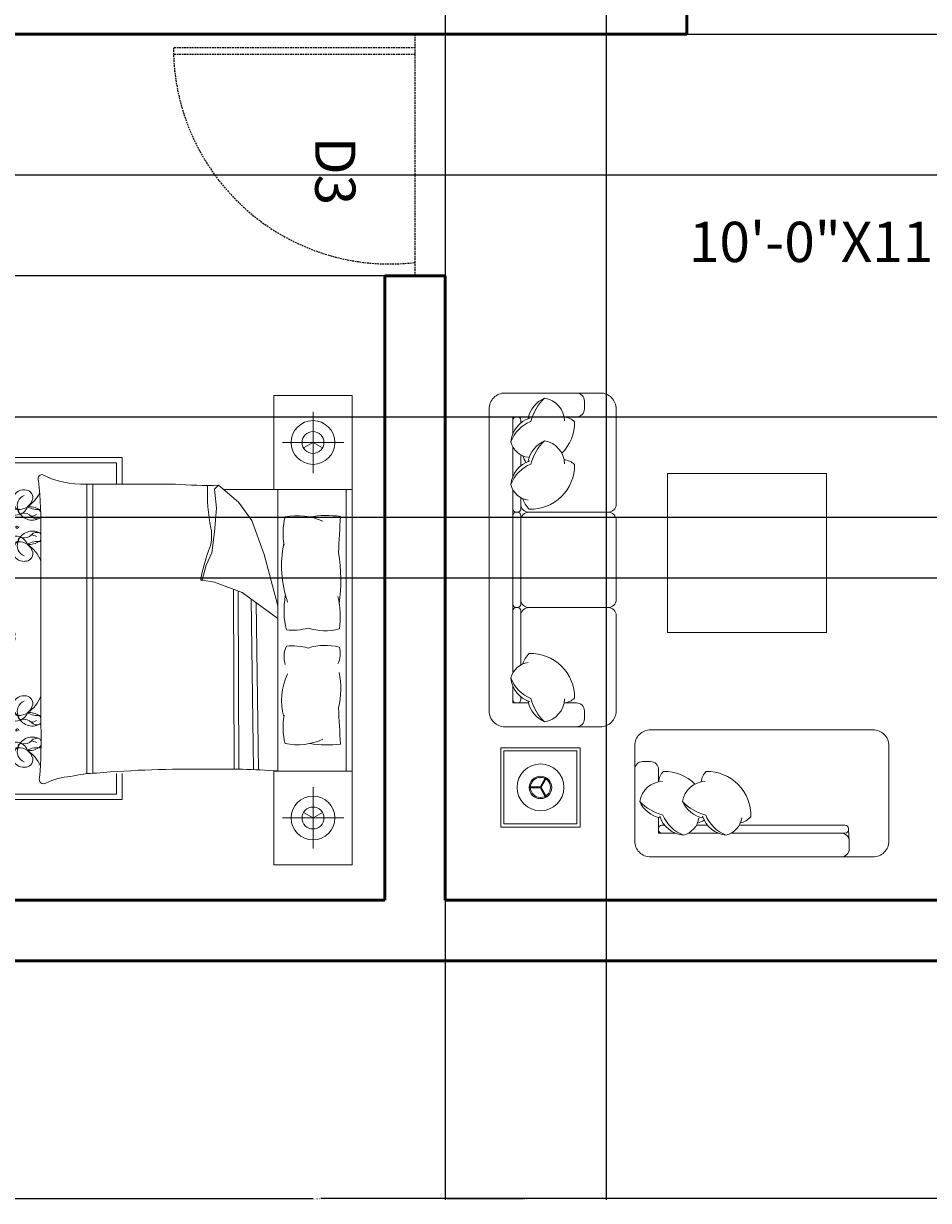
# Model space of a CAD drawing. Units: inches. Extents: x 3 to 576, y -689 to 51.
# Tile 3 of 21: x 201 to 336, y -689 to -514. Entities that reach past the tile are written whole.
import ezdxf

# ---------------------------------------------------------------- set-up
doc = ezdxf.new("R2010")
doc.units = ezdxf.units.IN
doc.header["$MEASUREMENT"] = 0
doc.linetypes.add('DASHED2', pattern=[0.375, 0.25, -0.125])
for name, color, linetype, lineweight in [('A-ANNO-DIMS', 2, 'Continuous', 18), ('A-ANNO-TEXT', 3, 'Continuous', 18), ('A-AREA-IDEN', 7, 'Continuous', 18), ('A-DOOR', 4, 'DASHED2', 25), ('A-FURN', 8, 'Continuous', 18), ('A-WALL', 7, 'Continuous', 50)]:
    doc.layers.add(name, color=color, linetype=linetype, lineweight=lineweight)
doc.styles.get("Standard").update_dxf_attribs({"font": 'arial.ttf'})
doc.dimstyles.get("Standard").update_dxf_attribs({"dimtxt": 0.18, "dimasz": 0.18, "dimexe": 0.18, "dimexo": 0.0625, "dimgap": 0.09, "dimtad": 0, "dimtih": 1, "dimtoh": 1, "dimdec": 0, "dimzin": 0, "dimdsep": 46, "dimlunit": 3, "dimtxsty": 'Standard', "dimcen": 0.09, "dimadec": 0, "dimazin": 0, "dimtfac": 1, "dimtdec": 0, "dimtofl": 0, "dimtmove": 0, "dimatfit": 3, "dimfxl": 1, "dimtolj": 1, "dimtzin": 0, "dimarcsym": 0})

# ---------------------------------------------------------------- blocks, each defined once
blk = doc.blocks.new('DAY BED1')
at = {"color": 0}
blk.add_line((0.3, 0.25), (0.225, 0.2549), dxfattribs=at)
blk.add_lwpolyline([(-0.3, 0, -0.414214), (-0.4, 0.1), (-0.4, 0.1, 0.317837), (-0.4, 0.1, -0.414214), (-0.4, 0.1), (-0.4, 0.1, 1.186185), (-0.4, 0.1, -0.414214), (-0.4, 0.1), (-0.4, 1.5, -0.414214), (-0.3, 1.6), (0.3, 1.6, -0.414214), (0.4, 1.5), (0.4, 0.1, -0.414214), (0.3, 0)], format="xyb", close=True, dxfattribs=at)
for points in [[(-0.0725, 1.45), (-0.15, 1.45, -0.414214), (-0.2, 1.5), (-0.2, 1.55, -0.414214), (-0.15, 1.6)], [(-0.0756, 1.4249, -0.356772), (0.0505, 1.5682, -0.249542), (0.1543, 1.4384, 9.61688)], [(0.0505, 1.5682, -0.14773), (0.1364, 1.422, -0.213343), (0.2624, 1.2931, -0.178662)], [(-0.0725, 1.4501, 0.165541), (-0.1386, 1.4192, 0.200231), (-0.0581, 1.2207, 0.121523)], [(0.1433, 1.4422, -0.306663), (0.2624, 1.2931, -0.30633), (0.1536, 1.1957, 0.872847)], [(0.25, 1.3448), (0.25, 1.45), (0.1517, 1.45, -0.414214)], [(0.2, 1.4118), (0.2, 1.43, -0.414214), (0.22, 1.45), (0.23, 1.45, -0.414214), (0.25, 1.43)], [(0.25, 1.43), (0.25, 1.3448, -0.414214)], [(-0.0756, 1.1556, -0.356772), (0.0505, 1.2988, -0.249542), (0.1543, 1.169, 9.61688)], [(0.0505, 1.2988, -0.14773), (0.1364, 1.1527, -0.213343), (0.2624, 1.0238, -0.178662)], [(0.25, 1.2616), (0.25, 1.0755, -0.414214)], [(0.1678, 1.1631, 0.071865), (0.1873, 1.205, -7.115464)], [(0.2, 1.1425), (0.2, 1.2113, -0.414214)], [(-0.0725, 1.1808, 0.165541), (-0.1386, 1.1498, 0.425989), (0.1479, 0.869, 0.121523), (0.1873, 0.9357, -7.115464)], [(0.1433, 1.1729, -0.306663), (0.2624, 1.0238, -0.30633), (0.1536, 0.9263, 0.872847)], [(0.25, 0.9923), (0.25, 0.2749, -0.414214), (0.23, 0.2549), (0.22, 0.2549, -0.414214), (0.2, 0.2749), (0.2, 0.9419, -0.414214)], [(0.25, 0.3775), (0.25, 0.3, 0.414214), (0.3, 0.25), (0.35, 0.25, 0.414214), (0.4, 0.3)]]:
    blk.add_lwpolyline(points, format="xyb", dxfattribs=at)
for points in [[(0.25, 1.0755), (0.25, 1.2616)], [(0.25, 0.3775), (0.25, 0.9923)]]:
    blk.add_lwpolyline(points, dxfattribs=at)
blk = doc.blocks.new('BED-DOUBLE')
for p, q in [((59.45, 69.91), (59.45, 0)), ((53.63, 58.35), (53.63, 67.49)), ((49.06, 62.92), (58.2, 62.92)), ((0, 60.68), (25.18, 60.68)), ((0, 9.72), (0, 60.68)), ((0.81, 59.87), (0.81, 10.53)), ((24.37, 59.87), (0.81, 59.87)), ((24.37, 56.73), (24.37, 59.87)), ((25.18, 60.68), (25.18, 56.73)), ((19.95, 13.6), (19.95, 56.73)), ((20.82, 13.66), (20.82, 56.73)), ((38.97, 55.99), (39.54, 56.55)), ((39.54, 56.55), (42.51, 54.01)), ((39.25, 53.16), (38.97, 55.99)), ((59.45, 55.93), (40.27, 55.93)), ((48.41, 55.93), (48.41, 13.98)), ((58.56, 13.98), (58.56, 55.93)), ((7.9, 52.98), (8.69, 53.14)), ((38.97, 49.62), (39.25, 53.16)), ((42.51, 54.01), (44.49, 51.31)), ((44.49, 51.31), (46.33, 46.22)), ((13.08, 20.76), (13.08, 49.15)), ((38.55, 46.5), (38.97, 49.62)), ((7.9, 48.1), (8.69, 47.94)), ((37.7, 44.66), (38.55, 46.5)), ((46.33, 46.22), (48.41, 38.59)), ((37.13, 42.39), (37.7, 44.66)), ((38.97, 42.11), (37.13, 42.39)), ((43.07, 40.55), (38.97, 42.11)), ((41.87, 14.23), (41.76, 41.05)), ((42.58, 14.23), (42.48, 40.78)), ((48.41, 36.72), (43.07, 40.55)), ((44.78, 14.2), (44.43, 39.58)), ((45.5, 14.17), (45.15, 39.06)), ((7.9, 22.3), (8.69, 22.46)), ((7.9, 17.41), (8.69, 17.26)), ((24.37, 10.53), (24.37, 13.61)), ((25.18, 13.59), (25.18, 9.72)), ((0.81, 10.53), (24.37, 10.53)), ((53.63, 11.56), (53.63, 2.42)), ((25.18, 9.72), (0, 9.72)), ((49.06, 6.99), (58.2, 6.99))]:
    blk.add_line(p, q)
for points in [[(47.8, 55.93), (47.8, 69.91), (59.45, 69.91)], [(53.63, 62.92), (52.22, 62.1)], [(53.63, 62.92), (55.04, 62.1)], [(59.45, 13.98), (47.8, 13.98), (47.8, 0), (59.45, 0)], [(53.63, 6.99), (52.22, 7.81)], [(53.63, 6.99), (55.04, 7.81)]]:
    blk.add_lwpolyline(points)
for points in [[(33.13, 56.7, 0.001242), (19.87, 56.73, -0.127202), (13.26, 58.14)], [(57.71, 51.91, 0.074897), (53.14, 51.83, -0.472817)], [(52.89, 35.28, 0.14099), (57.55, 35.14, 0.235245)], [(52.89, 32.3, -0.14099), (57.55, 32.44, -0.235245)], [(57.71, 18, -0.074897), (53.14, 18.08, 0.472817)], [(21.37, 13.68, 0.056112), (17.53, 13.18, 0.095341), (13.82, 12.19)]]:
    blk.add_lwpolyline(points, format="xyb")
for centre, radius in [((53.63, 62.92), 3.26), ((53.63, 62.92), 1.63), ((3.49, 50.11), 0.178), ((5.36, 48.94), 0.178), ((5.36, 21.45), 0.178), ((3.49, 20.29), 0.178), ((53.63, 6.99), 3.26), ((53.63, 6.99), 1.63)]:
    blk.add_circle(centre, radius)
for centre, radius, start, end in [((-2.47, 63.69), 5.54, 306.3036, 316.4814), ((-1.64, 62.09), 4.45, 303.4617, 330.1116), ((-0.42, 66.67), 9.13, 277.745, 311.8856), ((-1.32, 51.05), 9.13, 34.3865, 68.5908), ((13.3, 57.49), 0.645, 93.98, 207.3412), ((-0.61, 59.6), 3.71, 292.5547, 318.9546), ((1.38, 69.77), 12.63, 267.4081, 273.6519), ((6, 55.22), 1.01, 77.7115, 159.0387), ((5.45, 56.23), 0.762, 238.4633, 358.2869), ((7.95, 54.69), 2.31, 138.8402, 177.9352), ((6.56, 55.55), 0.747, 117.6827, 223.7762), ((6.39, 55.47), 0.757, 2.9516, 103.728), ((12.45, 57.59), 6.39, 192.5173, 207.1824), ((5.37, 55.04), 1.44, 345.4653, 54.2343), ((7.54, 57.02), 1.56, 211.3827, 255.2969), ((-59.69, 49.98), 72.78, 359.3433, 5.6887), ((37.8, 120.65), 64.12, 265.8294, 271.553), ((64.29, 55.36), 26.39, 177.4519, 191.3392), ((5.76, 54.77), 0.113, 177.9352, 11.4834), ((5.81, 54.78), 0.0551, 11.4834, 127.9409), ((6.09, 55.1), 0.0988, 223.7762, 159.7183), ((7.84, 54.58), 1.05, 350.264, 160.8688), ((8.16, 54.83), 1.31, 175.969, 254.3045), ((6.7, 54.8), 0.643, 333.9755, 53.2681), ((6.41, 53.42), 1.4, 6.1662, 51.5825), ((10.15, 56.66), 3.3, 211.2614, 251.7045), ((10.53, 54.2), 1.67, 84.9449, 172.8857), ((10.9, 54.49), 2.03, 182.3591, 234.0401), ((11.17, 53.54), 1.62, 111.5819, 201.4221), ((9.83, 55.04), 2.1, 265.2933, 346.921), ((10.7, 54.68), 1.18, 354.4856, 91.0538), ((8.16, 57.76), 5.29, 303.6671, 333.2997), ((9.88, 56.69), 3.75, 236.2883, 266.5076), ((9.4, 53.85), 1.74, 209.9085, 343.1337), ((10.13, 52.75), 0.434, 167.3041, 285.1471), ((11.31, 50.67), 2.7, 122.7011, 126.3445), ((11.81, 53.58), 2.23, 199.2822, 299.1751), ((12.57, 55.82), 2.9, 238.8218, 279.1554), ((11.31, 50.67), 2.7, 55.785, 94.7304), ((12.31, 52.24), 0.842, 30.0293, 52.325), ((3.75, 51.26), 0.199, 124.3538, 214.3923), ((4.04, 51.23), 0.464, 190.3057, 287.1958), ((4.17, 51.39), 0.538, 176.9701, 248.2913), ((8.01, 54.23), 5.2, 212.6784, 216.3746), ((3.99, 51.27), 0.206, 216.3746, 291.7548), ((2.83, 48.01), 3.1, 63.7819, 68.2913), ((4.48, 51.12), 0.464, 122.8155, 187.3992), ((4.12, 50.93), 0.155, 289.3605, 111.7548), ((4.24, 50.93), 0.155, 221.8703, 44.2646), ((4.69, 51.06), 0.538, 109.4799, 177.6828), ((4.4, 51.4), 0.199, 56.8636, 146.9021), ((4.5, 51.18), 0.206, 148.8844, 224.2646), ((8.78, 48.6), 5.2, 145.1882, 148.8844), ((5.81, 48.38), 2.9, 94.756, 119.2041), ((11.99, 44.2), 9.55, 132.2412, 142.1744), ((7.17, 51.8), 1.97, 178.3264, 187.1302), ((5.04, 51.53), 0.367, 11.3256, 64.4621), ((6.29, 52.06), 1.1, 190.2588, 210.656), ((5.55, 51.61), 0.336, 188.3432, 274.2869), ((5.84, 51.79), 0.586, 210.656, 242.6341), ((6.28, 52.3), 1.12, 218.2101, 226.3071), ((5.45, 51.35), 0.142, 325.7657, 67.4417), ((1.03, 56.11), 6.64, 313.1541, 322.0459), ((5.96, 45.49), 5.79, 73.5842, 93.8277), ((5.91, 52.13), 0.137, 142.4737, 265.053), ((6.09, 52.15), 0.294, 127.7621, 169.0403), ((5.94, 52.4), 0.414, 265.053, 338.3618), ((6.48, 51.84), 0.541, 113.4276, 137.6104), ((6.42, 52.4), 0.178, 183.2768, 356.7232), ((6.55, 52.07), 0.291, 139.7889, 227.6792), ((6.46, 51.97), 0.153, 227.6792, 350.3487), ((5.87, 52.08), 0.583, 353.0852, 15.7171), ((6.25, 52.01), 0.368, 350.3487, 43.6538), ((6.93, 52.39), 0.428, 198.7263, 262.5032), ((6.59, 52.19), 0.17, 1.1081, 91.8675), ((6.91, 52.1), 0.138, 255.2356, 54.9248), ((6.7, 52.15), 0.297, 11.5637, 52.6358), ((9.52, 51.39), 1.97, 178.3264, 187.1302), ((7.39, 51.11), 0.367, 11.3256, 64.4621), ((8.64, 51.64), 1.1, 190.2588, 210.656), ((7.9, 51.19), 0.336, 188.3432, 274.2869), ((8.19, 51.38), 0.586, 210.656, 242.6341), ((8.64, 51.88), 1.12, 218.2101, 226.3071), ((7.81, 50.93), 0.142, 325.7657, 67.4417), ((8.21, 50.67), 0.336, 147.5332, 233.4768), ((7.94, 50.71), 0.142, 354.3784, 96.0543), ((8.51, 50.85), 0.586, 179.1859, 211.164), ((5.96, 45.49), 5.79, 63.0032, 69.8941), ((10.62, 50.95), 1.43, 41.5653, 105.1471), ((11.41, 53.92), 2.01, 277.436, 299.9149), ((12.48, 52.59), 1.05, 221.5653, 293.8354), ((12.31, 52.24), 0.842, 314.4517, 333.558), ((58.53, 49.42), 9.37, 165.1039, 191.0369), ((51.31, 43.01), 9.01, 65.1316, 101.7583), ((723.03, 13.38), 666.43, 176.68521, 177.14978), ((2.98, 49.84), 0.137, 142.4737, 265.053), ((3.16, 49.87), 0.294, 61.2196, 169.0403), ((3, 50.12), 0.414, 265.053, 338.3618), ((3.35, 50.47), 0.351, 157.4086, 261.4386), ((3.15, 50.48), 0.176, 58.0499, 135.6268), ((3.55, 49.55), 0.541, 113.4276, 137.6104), ((3.34, 50.37), 0.118, 172.906, 277.132), ((2.95, 50.16), 0.561, 14.7558, 58.0499), ((3.62, 49.79), 0.291, 139.7889, 227.6792), ((3.53, 49.68), 0.153, 227.6792, 350.3487), ((3.74, 50.31), 0.243, 36.1046, 181.4281), ((2.93, 49.79), 0.583, 353.0852, 15.7171), ((3.31, 49.72), 0.368, 350.3487, 43.6538), ((3.59, 50.5), 0.245, 270.0645, 331.1507), ((3.8, 50.44), 0.28, 221.8413, 265.7877), ((4, 50.1), 0.428, 198.7263, 262.5032), ((3.66, 49.9), 0.17, 1.1081, 91.8675), ((3.8, 50.33), 0.174, 263.7526, 41.7054), ((3.76, 49.86), 0.297, 11.5637, 86.365), ((5.81, 48.38), 2.9, 124.0033, 132.4917), ((3.98, 49.81), 0.138, 255.2356, 54.9248), ((4.48, 50.4), 0.493, 128.3208, 208.8162), ((4.57, 50.43), 0.59, 207.7043, 254.3516), ((4.94, 50.48), 0.812, 157.2305, 229.0635), ((4.67, 50.75), 0.478, 174.4544, 220.6188), ((4.19, 50.1), 0.812, 270.278, 342.111), ((4.73, 49.08), 0.574, 98.7227, 159.3375), ((4.44, 49.82), 0.59, 244.9899, 291.6373), ((1.96, 48.08), 3.48, 30.544, 49.818), ((3.87, 50.06), 0.574, 340.0041, 40.6188), ((4.57, 50.12), 0.478, 278.7227, 324.8872), ((4.49, 49.73), 0.493, 290.5253, 358.5375), ((5.23, 49.31), 0.351, 157.4086, 261.4386), ((5.03, 49.32), 0.176, 58.0499, 135.6268), ((5.45, 49.87), 0.493, 182.8499, 266.1226), ((5.26, 50.22), 0.478, 231.7607, 277.9252), ((5.63, 50.31), 0.812, 214.5369, 286.3699), ((5.21, 49.21), 0.118, 172.906, 277.132), ((4.83, 48.99), 0.561, 14.7558, 58.0499), ((1.96, 48.08), 3.48, 23.0501, 23.8477), ((5.4, 49.18), 0.574, 37.3105, 97.9252), ((5.61, 49.14), 0.243, 36.1046, 181.4281), ((5.47, 49.97), 0.59, 265.0106, 311.658), ((5.47, 49.33), 0.245, 270.0645, 331.1507), ((5.68, 49.17), 0.174, 263.7526, 41.7054), ((8.95, 51.12), 1.1, 211.164, 231.5612), ((9.15, 52.01), 1.97, 234.6898, 243.4936), ((9.16, 51), 1.12, 195.5129, 203.6099), ((7.9, 50.27), 0.367, 357.3579, 50.4944), ((9.48, 50.34), 0.135, 12.7051, 190.4384), ((9.56, 50.36), 0.219, 190.4384, 10.4136), ((11.81, 47.5), 2.23, 60.8249, 160.7178), ((10.62, 50.13), 1.43, 254.8529, 318.4347), ((11.41, 47.16), 2.01, 60.0851, 82.564), ((12.48, 48.49), 1.05, 66.1646, 138.4347), ((12.31, 48.84), 0.842, 23.229, 45.5483), ((32.84, 49.05), 5.69, 336.2616, 11.3392), ((4.85, 48.67), 0.137, 142.4737, 265.053), ((5.03, 48.7), 0.294, 61.2196, 169.0403), ((4.88, 48.95), 0.414, 265.053, 338.3618), ((5.43, 48.38), 0.541, 113.4276, 137.6104), ((5.5, 48.62), 0.291, 139.7889, 227.6792), ((5.4, 48.52), 0.153, 227.6792, 350.3487), ((4.81, 48.63), 0.583, 353.0852, 15.7171), ((1.96, 48.08), 3.48, 357.1071, 4.7585), ((5.19, 48.56), 0.368, 350.3487, 43.6538), ((5.68, 49.27), 0.28, 221.8413, 265.7877), ((5.87, 48.94), 0.428, 198.7263, 262.5032), ((5.53, 48.74), 0.17, 1.1081, 91.8675), ((5.64, 48.7), 0.297, 11.5637, 86.365), ((5.85, 48.65), 0.138, 255.2356, 54.9248), ((8.16, 46.25), 1.31, 105.6955, 184.031), ((6.41, 47.66), 1.4, 308.4175, 353.8338), ((10.15, 44.42), 3.3, 108.2955, 148.7386), ((9.88, 44.39), 3.75, 93.4924, 123.7117), ((9.4, 47.23), 1.74, 16.8663, 150.0915), ((10.9, 46.59), 2.03, 125.9599, 177.6409), ((11.17, 47.54), 1.62, 158.5779, 248.4181), ((9.83, 46.04), 2.1, 13.079, 94.7067), ((10.13, 48.33), 0.434, 74.8529, 192.6959), ((11.31, 50.41), 2.7, 233.6555, 237.2989), ((12.57, 45.26), 2.9, 79.7133, 121.1782), ((11.31, 50.41), 2.7, 265.2696, 304.215), ((8.16, 43.32), 5.29, 21.4941, 56.3329), ((12.31, 48.84), 0.842, 307.675, 336.7144), ((65.19, 44.49), 16.25, 168.0397, 199.2615), ((5.45, 44.85), 0.762, 1.7131, 121.5367), ((5.76, 46.31), 0.113, 348.5166, 182.0648), ((7.95, 46.39), 2.31, 182.0648, 221.1598), ((5.81, 46.3), 0.0551, 232.0591, 348.5166), ((6.56, 45.54), 0.747, 136.2238, 242.3173), ((6.13, 45.97), 0.0595, 200.2667, 136.2271), ((5.37, 46.05), 1.44, 305.7657, 14.5347), ((12.45, 43.49), 6.39, 152.8176, 167.4827), ((7.84, 46.5), 1.05, 199.1312, 9.736), ((6.7, 46.28), 0.643, 306.7319, 26.0245), ((10.53, 46.88), 1.67, 187.1143, 275.0551), ((10.7, 46.4), 1.18, 268.9462, 5.5144), ((63.55, 37.54), 27.11, 160.1194, 169.3383), ((32.41, 42.33), 25.35, 352.2196, 9.497), ((-0.61, 41.48), 3.71, 41.0454, 67.4453), ((1.38, 31.32), 12.63, 86.3481, 92.5919), ((-1.32, 50.03), 9.13, 291.4092, 325.6135), ((6, 45.86), 1.01, 200.9613, 282.2885), ((6.39, 45.61), 0.757, 256.272, 357.0484), ((7.54, 44.06), 1.56, 104.7031, 148.6173), ((-0.42, 34.41), 9.13, 4.4623, 82.255), ((-1.64, 38.99), 4.45, 1.272, 56.5383), ((37.07, 42.55), 0.169, 178.8623, 289.7536), ((-2.47, 37.39), 5.54, 17.8504, 53.6964), ((-4.03, 34.48), 8.25, 34.0123, 54.053), ((-3.99, 37.66), 5.02, 343.5431, 17.0202), ((-5.31, 35.11), 9.13, 4.4623, 27.4146), ((61.64, 37.91), 12.33, 169.8617, 193.6238), ((45.23, 36.98), 12.46, 351.5249, 13.96), ((-6.58, 35.67), 7.42, 4.3787, 5.6357), ((-11.66, 31.77), 13.27, 19.7217, 19.9028), ((3.11, 35.07), 1.01, 47.7873, 129.1145), ((3.14, 36.22), 0.762, 208.5391, 328.3627), ((4.54, 33.64), 2.31, 108.9159, 148.011), ((3.76, 35.07), 0.747, 87.7585, 193.852), ((9.89, 33.91), 6.39, 162.593, 177.2582), ((2.48, 35.23), 1.44, 315.5411, 24.3101), ((5.35, 35.86), 1.56, 181.4585, 225.3727), ((3.58, 35.09), 0.757, 333.0274, 73.8037), ((8, 34.37), 1.01, 47.7873, 129.1145), ((8.03, 35.52), 0.762, 208.5391, 328.3627), ((9.43, 32.94), 2.31, 108.9159, 148.011), ((8.65, 34.38), 0.747, 87.7585, 193.852), ((7.37, 34.53), 1.44, 315.5411, 24.3101), ((14.78, 33.21), 6.39, 162.593, 177.2582), ((8.47, 34.4), 0.757, 333.0274, 73.8037), ((10.24, 35.16), 1.56, 181.4585, 225.3727), ((50.55, 43.52), 8.57, 264.0129, 285.8293), ((2.68, 34.8), 0.113, 148.011, 341.5592), ((2.68, 33.27), 0.113, 18.4408, 211.989), ((2.73, 34.78), 0.0551, 341.5592, 98.0167), ((3.13, 34.92), 0.0988, 193.852, 129.9245), ((9.89, 34.16), 6.39, 182.7418, 197.407), ((2.48, 32.84), 1.44, 335.6899, 44.4589), ((5.35, 32.21), 1.56, 134.6273, 178.5415), ((3.58, 32.97), 0.757, 286.1963, 26.9726), ((7.57, 34.1), 0.113, 148.011, 341.5592), ((7.57, 33.97), 0.113, 18.4408, 211.989), ((9.43, 35.13), 2.31, 211.989, 251.0841), ((7.62, 34.08), 0.0551, 341.5592, 98.0167), ((7.62, 33.99), 0.0551, 261.9833, 18.4408), ((8.65, 33.69), 0.747, 166.148, 272.2415), ((8.02, 34.22), 0.0988, 193.852, 129.9245), ((8.06, 33.86), 0.0595, 230.1909, 166.0209), ((7.37, 33.54), 1.44, 335.6899, 44.4589), ((14.78, 34.86), 6.39, 182.7418, 197.407), ((8.47, 33.67), 0.757, 286.1963, 26.9726), ((10.24, 32.91), 1.56, 134.6273, 178.5415), ((1.69, 33.95), 7.07, 262.8636, 351.8197), ((-3.99, 30.4), 5.02, 342.9798, 16.4569), ((-6.58, 32.39), 7.42, 354.3643, 355.6213), ((-11.66, 36.3), 13.27, 340.0972, 340.2783), ((3.14, 31.85), 0.762, 31.6373, 151.4609), ((3.11, 33), 1.01, 230.8855, 312.2127), ((4.54, 34.43), 2.31, 211.989, 251.0841), ((2.73, 33.29), 0.0551, 261.9833, 18.4408), ((-5.31, 32.96), 9.13, 332.5854, 355.5377), ((3.76, 32.99), 0.747, 166.148, 272.2415), ((3.17, 33.16), 0.0595, 230.1909, 166.0209), ((8.03, 32.55), 0.762, 31.6373, 151.4609), ((8, 33.7), 1.01, 230.8855, 312.2127), ((53.02, 31.01), 3.71, 155.0183, 198.5407), ((50.55, 24.06), 8.57, 74.1707, 95.9871), ((54.23, 31.48), 3.46, 333.3437, 16.1026), ((2.33, 33.04), 4.09, 248.117, 276.6195), ((1.2, 29.29), 1.64, 256.3898, 349.0739), ((1.42, 30.52), 2.07, 252.8609, 311.9049), ((-1.32, 20.37), 9.13, 34.3865, 68.5908), ((57.84, 24.53), 8.9, 153.8761, 196.1746), ((45.48, 26.29), 12.29, 346.3427, 11.1841), ((1.38, 39.08), 12.63, 267.4081, 273.6519), ((-0.61, 28.92), 3.71, 292.5547, 318.9546), ((6, 24.53), 1.01, 77.7115, 159.0387), ((5.45, 25.55), 0.762, 238.4633, 358.2869), ((7.95, 24), 2.31, 138.8402, 177.9352), ((6.56, 24.86), 0.747, 117.6827, 223.7762), ((6.39, 24.79), 0.757, 2.9516, 103.728), ((7.54, 26.34), 1.56, 211.3827, 255.2969), ((5.37, 24.35), 1.44, 345.4653, 54.2343), ((12.45, 26.91), 6.39, 192.5173, 207.1824), ((7.84, 23.9), 1.05, 350.264, 160.8688), ((6.7, 24.12), 0.643, 333.9755, 53.2681), ((10.53, 23.52), 1.67, 84.9449, 172.8857), ((10.7, 24), 1.18, 354.4856, 91.0538), ((8.16, 27.08), 5.29, 303.6671, 338.5059), ((5.76, 24.08), 0.113, 177.9352, 11.4834), ((5.81, 24.09), 0.0551, 11.4834, 127.9409), ((6.09, 24.41), 0.0988, 223.7762, 159.7183), ((8.16, 24.15), 1.31, 175.969, 254.3045), ((6.41, 22.74), 1.4, 6.1662, 51.5825), ((10.15, 25.98), 3.3, 211.2614, 251.7045), ((9.88, 26.01), 3.75, 236.2883, 266.5076), ((10.9, 23.81), 2.03, 182.3591, 234.0401), ((11.17, 22.86), 1.62, 111.5819, 201.4221), ((9.83, 24.36), 2.1, 265.2933, 346.921), ((723.03, 56.53), 666.43, 182.85022, 183.31479), ((4.44, 20.58), 0.59, 68.3627, 115.0101), ((4.19, 20.3), 0.812, 17.889, 89.722), ((4.73, 21.32), 0.574, 200.6625, 261.2773), ((4.49, 20.66), 0.493, 1.4625, 69.4747), ((4.85, 21.72), 0.137, 94.947, 217.5263), ((5.03, 21.7), 0.294, 190.9597, 298.7804), ((4.88, 21.45), 0.414, 21.6382, 94.947), ((5.23, 21.09), 0.351, 98.5614, 202.5914), ((5.43, 22.01), 0.541, 222.3896, 246.5724), ((5.21, 21.19), 0.118, 82.868, 187.094), ((4.83, 21.41), 0.561, 301.9501, 345.2442), ((5.5, 21.78), 0.291, 132.3208, 220.2111), ((5.4, 21.88), 0.153, 9.6513, 132.3208), ((4.81, 21.77), 0.583, 344.2829, 6.9148), ((5.61, 21.26), 0.243, 178.5719, 323.8954), ((1.96, 22.32), 3.48, 355.2415, 2.8929), ((5.19, 21.84), 0.368, 316.3462, 9.6513), ((5.87, 21.46), 0.428, 97.4968, 161.2737), ((5.68, 21.12), 0.28, 94.2123, 138.1587), ((5.47, 21.07), 0.245, 28.8493, 89.9355), ((5.53, 21.66), 0.17, 268.1325, 358.8919), ((5.64, 21.7), 0.297, 273.635, 348.4363), ((5.68, 21.23), 0.174, 318.2946, 96.2474), ((5.85, 21.75), 0.138, 305.0752, 104.7644), ((9.4, 23.17), 1.74, 209.9085, 343.1337), ((10.13, 22.07), 0.434, 167.3041, 285.1471), ((11.31, 19.99), 2.7, 122.7011, 126.3445), ((11.81, 22.9), 2.23, 199.2822, 299.1751), ((10.62, 20.26), 1.43, 41.5653, 105.1471), ((12.57, 25.14), 2.9, 238.8218, 280.2867), ((11.31, 19.99), 2.7, 55.785, 94.7304), ((11.41, 23.23), 2.01, 277.436, 299.9149), ((12.48, 21.91), 1.05, 221.5653, 293.8354), ((12.31, 21.55), 0.842, 23.2856, 52.325), ((12.31, 21.55), 0.842, 314.4517, 336.7144), ((58.53, 20.49), 9.37, 168.9631, 194.8961), ((2.98, 20.56), 0.137, 94.947, 217.5263), ((3.16, 20.53), 0.294, 190.9597, 298.7804), ((3, 20.28), 0.414, 21.6382, 94.947), ((3.35, 19.93), 0.351, 98.5614, 202.5914), ((3.15, 19.91), 0.176, 224.3732, 301.9501), ((3.55, 20.85), 0.541, 222.3896, 246.5724), ((3.34, 20.03), 0.118, 82.868, 187.094), ((2.95, 20.24), 0.561, 301.9501, 345.2442), ((3.62, 20.61), 0.291, 132.3208, 220.2111), ((3.53, 20.71), 0.153, 9.6513, 132.3208), ((2.93, 20.61), 0.583, 344.2829, 6.9148), ((3.74, 20.09), 0.243, 178.5719, 323.8954), ((3.31, 20.68), 0.368, 316.3462, 9.6513), ((4.04, 19.17), 0.464, 72.8042, 169.6943), ((4, 20.3), 0.428, 97.4968, 161.2737), ((3.8, 19.96), 0.28, 94.2123, 138.1587), ((3.59, 19.9), 0.245, 28.8493, 89.9355), ((4.17, 19.01), 0.538, 111.7087, 183.0299), ((3.66, 20.5), 0.17, 268.1325, 358.8919), ((3.76, 20.54), 0.297, 273.635, 348.4363), ((3.8, 20.07), 0.174, 318.2946, 96.2474), ((3.99, 19.13), 0.206, 68.2452, 143.6254), ((5.81, 22.02), 2.9, 227.5083, 235.9967), ((3.98, 20.59), 0.138, 305.0752, 104.7644), ((2.83, 22.39), 3.1, 291.7087, 296.2181), ((4.48, 20), 0.493, 151.1838, 231.6792), ((4.48, 19.27), 0.464, 172.6008, 237.1845), ((4.57, 19.96), 0.59, 105.6484, 152.2957), ((4.12, 19.47), 0.155, 248.2452, 70.6395), ((4.94, 19.92), 0.812, 130.9365, 202.7695), ((4.24, 19.47), 0.155, 315.7354, 138.1297), ((4.69, 19.33), 0.538, 182.3172, 250.5201), ((4.67, 19.65), 0.478, 139.3812, 185.5456), ((1.96, 22.32), 3.48, 310.182, 329.456), ((4.5, 19.21), 0.206, 135.7354, 211.1156), ((3.87, 20.33), 0.574, 319.3812, 19.9959), ((5.81, 22.02), 2.9, 240.7959, 265.244), ((11.99, 26.2), 9.55, 217.8256, 227.7588), ((4.57, 20.28), 0.478, 35.1128, 81.2773), ((5.03, 21.08), 0.176, 224.3732, 301.9501), ((5.45, 20.52), 0.493, 93.8774, 177.1501), ((5.63, 20.09), 0.812, 73.6301, 145.4631), ((5.26, 20.18), 0.478, 82.0748, 128.2393), ((1.96, 22.32), 3.48, 336.1523, 336.9499), ((5.4, 21.22), 0.574, 262.0748, 322.6895), ((5.47, 20.43), 0.59, 48.342, 94.9894), ((5.96, 24.9), 5.79, 266.1723, 286.4158), ((8.64, 18.76), 1.1, 149.344, 169.7412), ((7.9, 19.21), 0.336, 85.7131, 171.6568), ((8.19, 19.02), 0.586, 117.3659, 149.344), ((8.64, 18.52), 1.12, 133.6929, 141.7899), ((7.81, 19.46), 0.142, 292.5583, 34.2343), ((8.21, 19.72), 0.336, 126.5232, 212.4668), ((8.51, 19.55), 0.586, 148.836, 180.8141), ((7.94, 19.68), 0.142, 263.9457, 5.6216), ((5.96, 24.9), 5.79, 290.1059, 296.9968), ((8.95, 19.28), 1.1, 128.4388, 148.836), ((9.15, 18.38), 1.97, 116.5064, 125.3102), ((9.16, 19.4), 1.12, 156.3901, 164.4871), ((7.9, 20.13), 0.367, 309.5056, 2.6421), ((9.56, 20.04), 0.219, 349.5864, 169.5616), ((9.48, 20.06), 0.135, 169.5616, 347.2949), ((-54.91, 18.62), 68.03, 355.2402, 1.8035), ((3.75, 19.14), 0.199, 145.6077, 235.6462), ((8.01, 16.17), 5.2, 143.6254, 147.3216), ((4.4, 18.99), 0.199, 213.0979, 303.1364), ((8.78, 21.8), 5.2, 211.1156, 214.8118), ((6.29, 18.34), 1.1, 149.344, 169.7412), ((7.17, 18.6), 1.97, 172.8698, 181.6736), ((5.04, 18.87), 0.367, 295.5379, 348.6744), ((5.55, 18.79), 0.336, 85.7131, 171.6568), ((5.84, 18.61), 0.586, 117.3659, 149.344), ((6.28, 18.1), 1.12, 133.6929, 141.7899), ((5.45, 19.05), 0.142, 292.5583, 34.2343), ((1.03, 14.28), 6.64, 37.9541, 46.8459), ((5.91, 18.27), 0.137, 94.947, 217.5263), ((6.09, 18.24), 0.294, 190.9597, 232.2379), ((5.94, 18), 0.414, 21.6382, 94.947), ((6.48, 18.56), 0.541, 222.3896, 246.5724), ((6.42, 18), 0.178, 3.2768, 176.7232), ((6.55, 18.32), 0.291, 132.3208, 220.2111), ((6.46, 18.43), 0.153, 9.6513, 132.3208), ((5.87, 18.32), 0.583, 344.2829, 6.9148), ((6.25, 18.39), 0.368, 316.3462, 9.6513), ((6.93, 18.01), 0.428, 97.4968, 161.2737), ((6.59, 18.21), 0.17, 268.1325, 358.8919), ((6.91, 18.3), 0.138, 305.0752, 104.7644), ((6.7, 18.25), 0.297, 307.3642, 348.4363), ((9.52, 19.01), 1.97, 172.8698, 181.6736), ((7.39, 19.29), 0.367, 295.5379, 348.6744), ((9.4, 16.55), 1.74, 16.8663, 150.0915), ((10.9, 15.91), 2.03, 125.9599, 177.6409), ((10.13, 17.65), 0.434, 74.8529, 192.6959), ((11.81, 16.82), 2.23, 60.8249, 160.7178), ((11.31, 19.72), 2.7, 233.6555, 237.2989), ((10.62, 19.45), 1.43, 254.8529, 318.4347), ((11.41, 16.48), 2.01, 60.0851, 82.564), ((12.48, 17.81), 1.05, 66.1646, 138.4347), ((12.31, 18.16), 0.842, 307.675, 342.5814), ((12.31, 18.16), 0.842, 16.6343, 45.5483), ((51.31, 26.9), 9.01, 258.2417, 294.8684), ((8.16, 15.56), 1.31, 105.6955, 184.031), ((7.84, 15.82), 1.05, 199.1312, 9.736), ((6.7, 15.6), 0.643, 306.7319, 26.0245), ((6.41, 16.98), 1.4, 308.4175, 353.8338), ((10.15, 13.74), 3.3, 108.2955, 148.7386), ((9.88, 13.7), 3.75, 93.4924, 123.7117), ((10.53, 16.2), 1.67, 187.1143, 275.0551), ((11.17, 16.86), 1.62, 158.5779, 248.4181), ((9.83, 15.35), 2.1, 13.079, 94.7067), ((10.7, 15.72), 1.18, 268.9462, 5.5144), ((12.57, 14.57), 2.9, 79.249, 121.1782), ((11.31, 19.72), 2.7, 265.2696, 304.215), ((8.16, 12.63), 5.29, 23.6453, 56.3329), ((-0.61, 10.8), 3.71, 41.0454, 67.4453), ((-1.32, 19.35), 9.13, 291.4092, 325.6135), ((5.45, 14.17), 0.762, 1.7131, 121.5367), ((6, 15.18), 1.01, 200.9613, 282.2885), ((5.76, 15.63), 0.113, 348.5166, 182.0648), ((7.95, 15.71), 2.31, 182.0648, 221.1598), ((5.81, 15.62), 0.0551, 232.0591, 348.5166), ((6.56, 14.85), 0.747, 136.2238, 242.3173), ((6.13, 15.29), 0.0595, 200.2667, 136.2271), ((12.45, 12.81), 6.39, 152.8176, 167.4827), ((5.37, 15.36), 1.44, 305.7657, 14.5347), ((7.54, 13.38), 1.56, 104.7031, 148.6173), ((6.39, 14.93), 0.757, 256.272, 357.0484), ((35.29, -149.59), 163.86, 89.1145, 94.8735), ((39.86, -111.34), 125.62, 86.1, 90.9282), ((1.38, 0.63), 12.63, 86.3481, 92.5919), ((-0.42, 3.73), 9.13, 48.1144, 82.255), ((13.47, 12.72), 0.637, 156.5219, 303.8264), ((-1.64, 8.31), 4.45, 29.8884, 56.5383), ((-2.47, 6.71), 5.54, 43.5186, 53.6964)]:
    blk.add_arc(centre, radius, start, end)
blk = doc.blocks.new('DOOR-900')
for p, q in [((34, 36), (0, 36)), ((2, 36), (2, 0)), ((36, 36), (34, 36))]:
    blk.add_line(p, q)
blk.add_arc((2, 32.22), 32.22, 270, 6.7329)
blk = doc.blocks.new('*D50')
at = {"layer": 'A-ANNO-DIMS', "color": 0, "lineweight": -2, "transparency": 16777216}
for p, q in [((388.02, -644.37), (388.02, -688.94)), ((102.29, -653.37), (102.29, -688.94)), ((102.47, -688.76), (244.55, -688.76)), ((387.84, -688.76), (245.77, -688.76))]:
    blk.add_line(p, q, dxfattribs=at)
at = {"layer": 'A-ANNO-DIMS', "color": 0, "transparency": 16777216}
for points in [[(102.47, -688.73), (102.47, -688.79), (102.29, -688.76)], [(387.84, -688.73), (387.84, -688.79), (388.02, -688.76)]]:
    blk.add_solid(points, dxfattribs=at)
at = {"layer": 'Defpoints', "color": 0, "transparency": 16777216}
for p in [(388.02, -644.31), (102.29, -653.31), (388.02, -688.76)]:
    blk.add_point(p, dxfattribs=at)
at = {"layer": 'A-ANNO-DIMS', "color": 0, "transparency": 16777216, "insert": (245.16, -688.76), "char_height": 0.18, "attachment_point": 5}
blk.add_mtext('\\A1;23\'-9 1/2"', dxfattribs=at)
blk = doc.blocks.new('*D73')
at = {"layer": 'A-ANNO-DIMS', "color": 0, "lineweight": -2, "transparency": 16777216}
for p, q in [((531.23, -449.31), (2.66, -449.31)), ((2.84, -449.49), (2.84, -518.13)), ((2.84, -587.13), (2.84, -518.49)), ((531.23, -587.31), (2.66, -587.31))]:
    blk.add_line(p, q, dxfattribs=at)
at = {"layer": 'A-ANNO-DIMS', "color": 0, "transparency": 16777216}
for points in [[(2.81, -449.49), (2.87, -449.49), (2.84, -449.31)], [(2.81, -587.13), (2.87, -587.13), (2.84, -587.31)]]:
    blk.add_solid(points, dxfattribs=at)
at = {"layer": 'Defpoints', "color": 0, "transparency": 16777216}
for p in [(531.29, -449.31), (2.84, -587.31), (531.29, -587.31)]:
    blk.add_point(p, dxfattribs=at)
at = {"layer": 'A-ANNO-DIMS', "color": 0, "transparency": 16777216, "insert": (2.84, -518.31), "char_height": 0.18, "attachment_point": 5}
blk.add_mtext('\\A1;11\'-6"', dxfattribs=at)
blk = doc.blocks.new('*D74')
at = {"layer": 'A-ANNO-DIMS', "color": 0, "lineweight": -2, "transparency": 16777216}
for p, q in [((531.23, -587.31), (2.66, -587.31)), ((2.84, -587.49), (2.84, -591.63)), ((2.84, -596.13), (2.84, -591.99)), ((540.23, -596.31), (2.66, -596.31))]:
    blk.add_line(p, q, dxfattribs=at)
at = {"layer": 'A-ANNO-DIMS', "color": 0, "transparency": 16777216}
for points in [[(2.81, -587.49), (2.87, -587.49), (2.84, -587.31)], [(2.81, -596.13), (2.87, -596.13), (2.84, -596.31)]]:
    blk.add_solid(points, dxfattribs=at)
at = {"layer": 'Defpoints', "color": 0, "transparency": 16777216}
for p in [(531.29, -587.31), (2.84, -596.31), (540.29, -596.31)]:
    blk.add_point(p, dxfattribs=at)
at = {"layer": 'A-ANNO-DIMS', "color": 0, "transparency": 16777216, "insert": (2.84, -591.81), "char_height": 0.18, "attachment_point": 5}
blk.add_mtext('\\A1;0\'-9"', dxfattribs=at)
blk = doc.blocks.new('*D93')
at = {"layer": 'A-ANNO-DIMS', "color": 0, "lineweight": -2, "transparency": 16777216}
for p, q in [((174.14, -515.31), (575.92, -515.31)), ((575.74, -515.49), (575.74, -525.59)), ((575.74, -536.06), (575.74, -525.96)), ((174.14, -536.24), (575.92, -536.24))]:
    blk.add_line(p, q, dxfattribs=at)
at = {"layer": 'A-ANNO-DIMS', "color": 0, "transparency": 16777216}
for points in [[(575.71, -515.49), (575.77, -515.49), (575.74, -515.31)], [(575.71, -536.06), (575.77, -536.06), (575.74, -536.24)]]:
    blk.add_solid(points, dxfattribs=at)
at = {"layer": 'Defpoints', "color": 0, "transparency": 16777216}
for p in [(174.08, -515.31), (174.08, -536.24), (575.74, -536.24)]:
    blk.add_point(p, dxfattribs=at)
at = {"layer": 'A-ANNO-DIMS', "color": 0, "transparency": 16777216, "insert": (575.74, -525.77), "char_height": 0.18, "attachment_point": 5}
blk.add_mtext('\\A1;1\'-9"', dxfattribs=at)
blk = doc.blocks.new('*D107')
at = {"layer": 'A-ANNO-DIMS', "color": 0, "lineweight": -2, "transparency": 16777216}
for p, q in [((111.36, -515.31), (575.92, -515.31)), ((575.74, -515.49), (575.74, -543.63)), ((575.74, -572.13), (575.74, -543.99)), ((111.36, -572.31), (575.92, -572.31))]:
    blk.add_line(p, q, dxfattribs=at)
at = {"layer": 'A-ANNO-DIMS', "color": 0, "transparency": 16777216}
for points in [[(575.71, -515.49), (575.77, -515.49), (575.74, -515.31)], [(575.71, -572.13), (575.77, -572.13), (575.74, -572.31)]]:
    blk.add_solid(points, dxfattribs=at)
at = {"layer": 'Defpoints', "color": 0, "transparency": 16777216}
for p in [(111.29, -515.31), (111.29, -572.31), (575.74, -572.31)]:
    blk.add_point(p, dxfattribs=at)
at = {"layer": 'A-ANNO-DIMS', "color": 0, "transparency": 16777216, "insert": (575.74, -543.81), "char_height": 0.18, "attachment_point": 5}
blk.add_mtext('\\A1;4\'-9"', dxfattribs=at)
blk = doc.blocks.new('*D109')
at = {"layer": 'A-ANNO-DIMS', "color": 0, "lineweight": -2, "transparency": 16777216}
for p, q in [((255.23, -551.31), (2.66, -551.31)), ((2.84, -551.49), (2.84, -597.63)), ((2.84, -644.13), (2.84, -597.99)), ((255.23, -644.31), (2.66, -644.31))]:
    blk.add_line(p, q, dxfattribs=at)
at = {"layer": 'A-ANNO-DIMS', "color": 0, "transparency": 16777216}
for points in [[(2.81, -551.49), (2.87, -551.49), (2.84, -551.31)], [(2.81, -644.13), (2.87, -644.13), (2.84, -644.31)]]:
    blk.add_solid(points, dxfattribs=at)
at = {"layer": 'Defpoints', "color": 0, "transparency": 16777216}
for p in [(255.29, -551.31), (2.84, -644.31), (255.29, -644.31)]:
    blk.add_point(p, dxfattribs=at)
at = {"layer": 'A-ANNO-DIMS', "color": 0, "transparency": 16777216, "insert": (2.84, -597.81), "char_height": 0.18, "attachment_point": 5}
blk.add_mtext('\\A1;7\'-9"', dxfattribs=at)
blk = doc.blocks.new('*D115')
at = {"layer": 'A-ANNO-DIMS', "color": 0, "lineweight": -2, "transparency": 16777216}
for p, q in [((264.29, -134.37), (264.29, -688.94)), ((288.29, -134.37), (288.29, -688.94)), ((264.47, -688.76), (275.96, -688.76)), ((288.11, -688.76), (276.62, -688.76))]:
    blk.add_line(p, q, dxfattribs=at)
at = {"layer": 'A-ANNO-DIMS', "color": 0, "transparency": 16777216}
for points in [[(264.47, -688.73), (264.47, -688.79), (264.29, -688.76)], [(288.11, -688.73), (288.11, -688.79), (288.29, -688.76)]]:
    blk.add_solid(points, dxfattribs=at)
at = {"layer": 'Defpoints', "color": 0, "transparency": 16777216}
for p in [(264.29, -134.31), (288.29, -134.31), (288.29, -688.76)]:
    blk.add_point(p, dxfattribs=at)
at = {"layer": 'A-ANNO-DIMS', "color": 0, "transparency": 16777216, "insert": (276.29, -688.76), "char_height": 0.18, "attachment_point": 5}
blk.add_mtext('\\A1;2\'-0"', dxfattribs=at)

msp = doc.modelspace()

# ---------------------------------------------------------------- linework, layer by layer
at = {"layer": 'A-DOOR'}
msp.add_line((259.79, -518.31), (223.79, -518.31), dxfattribs=at)
at = {"layer": 'A-FURN'}
for p, q in [((278.48, -627.42), (276.81, -627.42)), ((278.48, -627.57), (276.81, -627.57)), ((278.42, -627.46), (279.25, -626.01)), ((278.42, -627.53), (279.25, -628.98)), ((278.54, -627.53), (279.38, -626.09)), ((278.54, -627.46), (279.38, -628.91))]:
    msp.add_line(p, q, dxfattribs=at)
at = {"layer": 'A-FURN', "ltscale": 0.03}
msp.add_lwpolyline([(287.39, -618.47, 0.414214), (289.76, -616.1), (289.76, -601.9, 0.414214), (288.57, -600.71, 0.414214), (289.76, -599.53), (289.76, -587.69, 0.414214), (288.57, -586.51, 0.414214), (289.76, -585.33), (289.76, -571.12, 0.414214), (287.39, -568.75), (273.19, -568.75, 0.414214), (270.82, -571.12), (270.82, -616.1, 0.414214), (273.19, -618.47)], format="xyb", close=True, dxfattribs=at)
at = {"layer": 'A-FURN'}
for points in [[(279.09, -569.51, 0.14773), (277.06, -572.97, 0.213343), (274.07, -576.02, 0.178662)], [(282.08, -572.9, 0.356772), (279.09, -569.51, 0.249542), (276.63, -572.58, -9.61688)], [(282, -572.31), (283.84, -572.31, 0.414214), (285.02, -571.12), (285.02, -569.94, 0.414214), (283.84, -568.75)], [(276.9, -572.49, 0.306663), (274.07, -576.02, 0.30633), (276.65, -578.33, -0.872847)], [(274.37, -574.8), (274.37, -572.31), (276.7, -572.31, 0.414214)], [(275.55, -573.21), (275.55, -572.78, 0.414214), (275.08, -572.31), (274.84, -572.31, 0.414214), (274.37, -572.78)], [(274.37, -572.78), (274.37, -574.8, 0.414214)], [(282, -572.3, -0.165541), (283.57, -573.03, -0.200231), (281.66, -577.73, -0.121523)], [(279.09, -575.88, 0.14773), (277.06, -579.34, 0.213343), (274.07, -582.4, 0.178662)], [(274.37, -576.76), (274.37, -581.17, 0.414214)], [(282.08, -579.28, 0.356772), (279.09, -575.88, 0.249542), (276.63, -578.96, -9.61688)], [(275.55, -579.59), (275.55, -577.96, 0.414214)], [(276.32, -579.1, -0.071865), (275.85, -578.1, 7.115464)], [(276.9, -578.87, 0.306663), (274.07, -582.4, 0.30633), (276.65, -584.7, -0.872847)], [(282, -578.68, -0.165541), (283.57, -579.41, -0.425989), (276.79, -586.06, -0.121523), (275.85, -584.48, 7.115464)], [(274.37, -583.14), (274.37, -586.04, 0.414214), (274.84, -586.51), (275.08, -586.51, 0.414214), (275.55, -586.04), (275.55, -584.33, 0.414214)], [(275.55, -585.33, 0.414214), (276.74, -586.51), (288.57, -586.51, 0.414214)], [(275.55, -587.69, -0.414214), (276.74, -586.51)], [(275.55, -599.53, 0.414214), (276.74, -600.71)], [(274.37, -610.46), (274.37, -601.19, -0.414214), (274.84, -600.71), (275.08, -600.71, -0.414214), (275.55, -601.19), (275.55, -609.27, -0.414214)], [(275.55, -601.9, -0.414214), (276.74, -600.71), (288.57, -600.71, -0.414214)], [(282, -614.92, 0.165541), (283.57, -614.19, 0.425989), (276.79, -607.54, 0.121523), (275.85, -609.12, -7.115464)], [(276.9, -614.73, -0.306663), (274.07, -611.2, -0.30633), (276.65, -608.9, 0.872847)], [(279.09, -617.72, -0.14773), (277.06, -614.26, -0.213343), (274.07, -611.2, -0.178662)], [(274.37, -614.44), (274.37, -612.43, -0.414214)], [(275.55, -614.01), (275.55, -614.44, -0.414214), (275.08, -614.92), (274.84, -614.92, -0.414214), (274.37, -614.44)], [(282.08, -614.32, -0.356772), (279.09, -617.72, -0.249542), (276.63, -614.64, 9.61688)], [(283.84, -618.47, 0.414214), (285.02, -617.29), (285.02, -616.1, 0.414214), (283.84, -614.92), (282, -614.92)]]:
    msp.add_lwpolyline(points, format="xyb", dxfattribs=at)
for points in [[(274.37, -581.17), (274.37, -576.76)], [(274.37, -610.46), (274.37, -583.14)], [(276.7, -614.92), (274.37, -614.92), (274.37, -612.43)]]:
    msp.add_lwpolyline(points, dxfattribs=at)
at = {"layer": 'A-FURN', "ltscale": 0.03}
for points in [[(321.09, -580.74), (321.09, -604.42), (297.42, -604.42), (297.42, -580.74)], [(284.4, -633.42), (284.4, -621.58), (272.56, -621.58), (272.56, -633.42)]]:
    msp.add_lwpolyline(points, close=True, dxfattribs=at)
at = {"layer": 'A-FURN'}
msp.add_lwpolyline([(274.37, -586.98), (274.37, -600.24, 0.414214), (274.84, -600.71), (275.08, -600.71, 0.414214), (275.55, -600.24), (275.55, -586.98, 0.414214), (275.08, -586.51), (274.84, -586.51, 0.414214)], format="xyb", close=True, dxfattribs=at)
msp.add_lwpolyline([(283.92, -622.05), (283.92, -632.94), (273.03, -632.94), (273.03, -622.05)], close=True, dxfattribs=at)
for radius in [3.49, 1.67, 1.5]:
    msp.add_circle((278.48, -627.5), radius, dxfattribs=at)
at = {"layer": 'A-WALL'}
for p, q in [((300.29, -506.31), (300.29, -515.31)), ((111.29, -515.31), (300.29, -515.31)), ((255.29, -551.31), (255.29, -644.31)), ((255.29, -551.31), (264.29, -551.31)), ((264.29, -551.31), (264.29, -644.31)), ((111.29, -644.31), (255.29, -644.31)), ((264.29, -644.31), (388.02, -644.31)), ((38.29, -653.31), (540.29, -653.31))]:
    msp.add_line(p, q, dxfattribs=at)

# ---------------------------------------------------------------- block references
at = {"layer": 'A-DOOR', "rotation": 270}
msp.add_blockref('DOOR-900', (223.79, -515.31), dxfattribs=at)
at = {"layer": 'A-FURN'}
msp.add_blockref('BED-DOUBLE', (190.96, -639.04), dxfattribs=at)
at = {"layer": 'A-FURN', "ltscale": 0.03, "xscale": -23.67362204300716, "yscale": 23.67362204300716, "zscale": 23.67362204300716, "rotation": 90}
msp.add_blockref('DAY BED1', (330.4, -628.39), dxfattribs=at)

# ---------------------------------------------------------------- texts
at = {"layer": 'A-ANNO-TEXT', "insert": (250.91, -530.59), "char_height": 6, "attachment_point": 1, "rotation": 270}
msp.add_mtext('D3', dxfattribs=at)
at = {"layer": 'A-AREA-IDEN', "insert": (300.61, -543.24), "char_height": 6, "attachment_point": 1}
msp.add_mtext('10\'-0"X11\'-0"', dxfattribs=at)

# ---------------------------------------------------------------- dimensions: what is measured, and where the dimension line sits
at = {"layer": 'A-ANNO-DIMS'}
for base, p1, p2, picture, middle in [((288.29, -688.76), (264.29, -134.31), (288.29, -134.31), '*D115', (276.29, -688.76)), ((388.02, -688.76), (102.29, -653.31), (388.02, -644.31), '*D50', (245.16, -688.76))]:
    dim = msp.add_linear_dim(base=base, p1=p1, p2=p2, dimstyle='Standard', override={"dimdec": 1, "dimlfac": 1, "dimrnd": 0, "dimzin": 1, "dimdsep": 46, "dimlunit": 4, "dimfrac": 2}, dxfattribs=at)
    dim.commit()
    dim.dimension.update_dxf_attribs({"geometry": picture, "text_midpoint": middle})
for base, p1, p2, picture, middle in [((2.84, -587.31), (531.29, -449.31), (531.29, -587.31), '*D73', (2.84, -518.31)), ((575.74, -572.31), (111.29, -515.31), (111.29, -572.31), '*D107', (575.74, -543.81)), ((575.74, -536.24), (174.08, -515.31), (174.08, -536.24), '*D93', (575.74, -525.77)), ((2.84, -644.31), (255.29, -551.31), (255.29, -644.31), '*D109', (2.84, -597.81)), ((2.84, -596.31), (531.29, -587.31), (540.29, -596.31), '*D74', (2.84, -591.81))]:
    dim = msp.add_linear_dim(base=base, p1=p1, p2=p2, angle=90, dimstyle='Standard', override={"dimdec": 1, "dimlfac": 1, "dimrnd": 0, "dimzin": 1, "dimdsep": 46, "dimlunit": 4, "dimfrac": 2}, dxfattribs=at)
    dim.commit()
    dim.dimension.update_dxf_attribs({"geometry": picture, "text_midpoint": middle})

doc.saveas('drawing.dxf')
